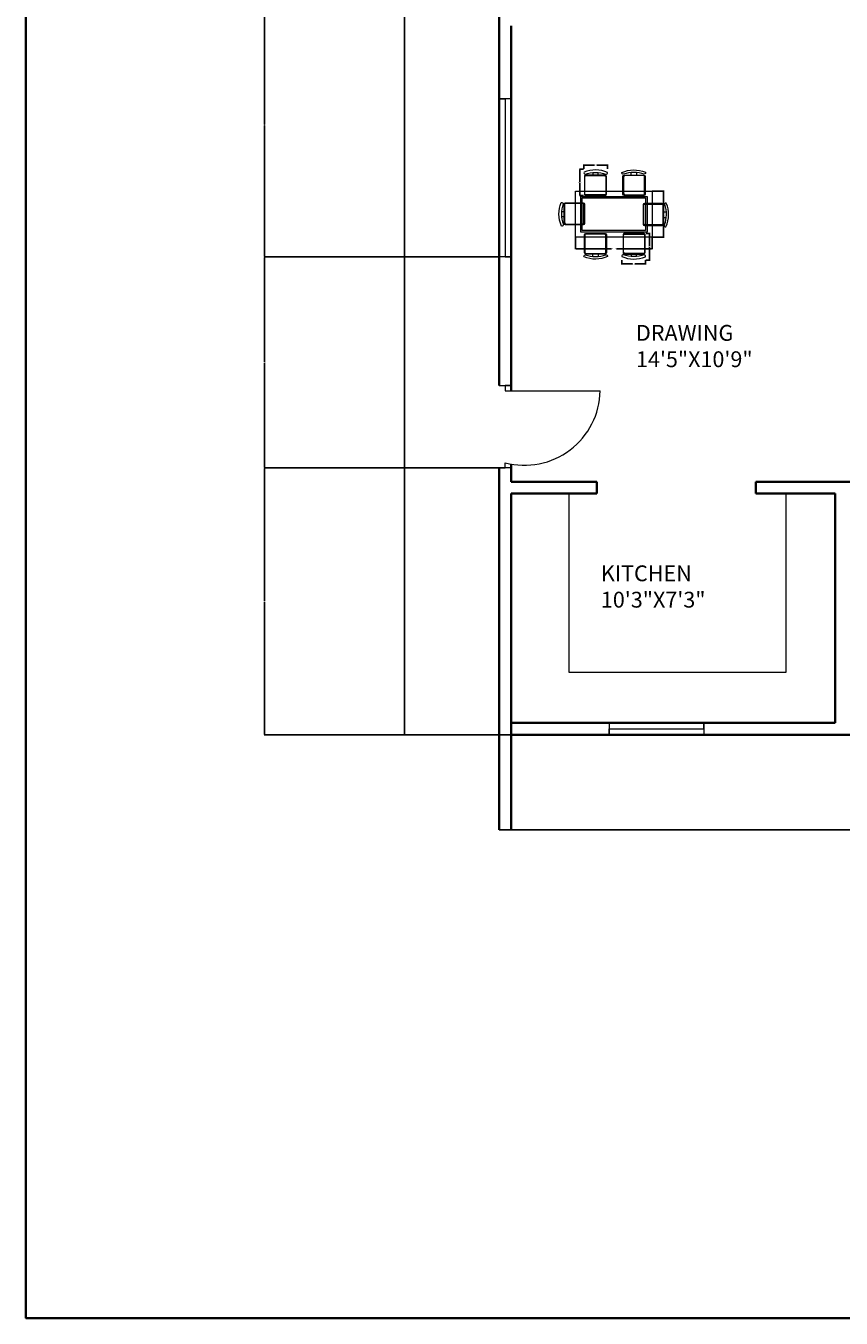
# Model space of a CAD drawing. Units: inches. Extents: x 1520 to 3401, y 1570 to 3432.
# Tile 1 of 15: x 1520 to 1829, y 1570 to 2061. Entities that reach past the tile are written whole.
import ezdxf

# ---------------------------------------------------------------- set-up
doc = ezdxf.new("R2010")
doc.units = ezdxf.units.IN
for name, color, linetype, lineweight in [('A-ANNO-DIMS', 2, 'Continuous', 18), ('A-ANNO-TTLB', 7, 'Continuous', 35), ('A-AREA-IDEN', 7, 'Continuous', 18), ('A-DOOR', 3, 'Continuous', 18), ('A-FLOR-CASE', 8, 'Continuous', 18), ('A-FLOR-EDGE', 7, 'Continuous', 25), ('A-FURN', 8, 'Continuous', 13), ('A-GLAZ', 4, 'Continuous', 18), ('A-WALL', 7, 'Continuous', 35)]:
    doc.layers.add(name, color=color, linetype=linetype, lineweight=lineweight)
doc.styles.get("Standard").update_dxf_attribs({"font": 'arial.ttf'})
doc.dimstyles.get("Standard").update_dxf_attribs({"dimtxt": 0.18, "dimasz": 0.18, "dimexe": 0.18, "dimexo": 0.0625, "dimgap": 0.09, "dimtad": 0, "dimtih": 1, "dimtoh": 1, "dimdec": 4, "dimzin": 0, "dimdsep": 46, "dimtxsty": 'Standard', "dimcen": 0.09, "dimadec": 0, "dimazin": 0, "dimtfac": 1, "dimtdec": 4, "dimtofl": 0, "dimtmove": 0, "dimatfit": 3, "dimfxl": 1, "dimtolj": 1, "dimtzin": 0, "dimarcsym": 0})

# ---------------------------------------------------------------- blocks, each defined once
blk = doc.blocks.new('DOOR-SWING-36-26')
for p, q in [((0, 31.26), (4.5, 31.26)), ((4.5, 31.26), (2.25, 31.26)), ((2.25, 31.26), (2.25, 29.26)), ((2.25, 29.26), (38.25, 29.26)), ((2.25, 0), (2.25, 2)), ((4.5, 0), (0, 0)), ((0, 0), (2.25, 0))]:
    blk.add_line(p, q)
blk.add_arc((9.61, 29.68), 28.64, 255.1135, 359.1603)
blk = doc.blocks.new('WIN-PLAN-60-02')
for p, q in [((4.5, 60), (0, 60)), ((0, 60), (2.25, 60)), ((2.25, 60), (2.25, 0)), ((4.5, 0), (0, 0)), ((2.25, 0), (4.5, 0))]:
    blk.add_line(p, q)
blk = doc.blocks.new('WIN-PLAN-36-04')
for p, q in [((0, 4.5), (0, 0)), ((0, 0), (0, 2.25)), ((0, 2.25), (36, 2.25)), ((36, 2.25), (36, 4.5)), ((36, 4.5), (36, 0))]:
    blk.add_line(p, q)
blk = doc.blocks.new('KITCHEN-COUNTER-01')
for p, q in [((0, 67.75), (0, 0)), ((82.51, 0), (82.51, 67.75)), ((0, 0), (82.51, 0))]:
    blk.add_line(p, q)
blk = doc.blocks.new('DINING-CHAIR-01')
for points in [[(0.47, 8.09, -0.175809), (8.38, 8.03, 0.578392), (8.97, 8.69, 0.214524), (0.06, 8.81, 0.552014), (0.47, 8.09, -0.065079)], [(8.04, 7.77), (0.7, 7.77, 0.414214), (0.19, 7.26), (0.19, 0.51, 0.414214), (0.7, 0), (8.04, 0, 0.414214), (8.55, 0.51), (8.55, 7.26, 0.414214), (8.04, 7.77)], [(5.46, 7.77), (5.46, 8.7, -0.064759)]]:
    blk.add_lwpolyline(points, format="xyb")
blk.add_lwpolyline([(0.71, 7.54), (7.81, 7.54, -0.414214), (8.32, 7.03), (8.32, 0.74, -0.414214), (7.81, 0.23), (0.71, 0.23, -0.512069), (0.42, 0.74), (0.42, 7.03, -0.512069)], format="xyb", close=True)
blk.add_lwpolyline([(3.41, 8.72), (3.41, 7.77)])
blk = doc.blocks.new('DINING-CHAIR-06')
for points in [[(8.29, 1.93, 0.414214), (8.81, 2.45), (8.81, 9.19, 0.414214), (8.29, 9.7), (0.96, 9.7, 0.414214), (0.45, 9.19), (0.45, 2.45, 0.414214), (0.96, 1.93), (8.29, 1.93)], [(8.52, 1.62, -0.175809), (0.62, 1.68, 0.578392), (0.02, 1.02, 0.214524), (8.94, 0.9, 0.552014), (8.52, 1.62, -0.065079)], [(3.53, 1.93), (3.53, 1, -0.064759)]]:
    blk.add_lwpolyline(points, format="xyb")
blk.add_lwpolyline([(8.29, 2.16), (1.19, 2.16, -0.414214), (0.68, 2.68), (0.68, 8.96, -0.414214), (1.19, 9.47), (8.29, 9.47, -0.512069), (8.58, 8.96), (8.58, 2.68, -0.512069)], format="xyb", close=True)
blk.add_lwpolyline([(5.59, 0.99), (5.59, 1.93)])
blk = doc.blocks.new('DINING-TABLE')
for points in [[(0, 17.41), (29.01, 17.41), (29.01, 0), (0, 0)], [(1.93, 15.47), (27.08, 15.47), (27.08, 1.93), (1.93, 1.93)], [(2.51, 14.89), (26.5, 14.89), (26.5, 2.51), (2.51, 2.51)]]:
    blk.add_lwpolyline(points, close=True)
blk = doc.blocks.new('*D175')
at = {"layer": 'A-ANNO-DIMS', "color": 0, "lineweight": -2, "transparency": 16777216}
for p, q in [((1731.63, 2006.36), (1730, 2006.36)), ((1730.18, 2006.18), (1730.18, 2001.52)), ((1730.18, 1996.49), (1730.18, 2001.15)), ((1731.63, 1996.31), (1730, 1996.31))]:
    blk.add_line(p, q, dxfattribs=at)
at = {"layer": 'A-ANNO-DIMS', "color": 0, "transparency": 16777216}
for points in [[(1730.15, 2006.18), (1730.21, 2006.18), (1730.18, 2006.36)], [(1730.15, 1996.49), (1730.21, 1996.49), (1730.18, 1996.31)]]:
    blk.add_solid(points, dxfattribs=at)
at = {"layer": 'Defpoints', "color": 0, "transparency": 16777216}
for p in [(1730.18, 2006.36), (1731.69, 2006.36), (1731.69, 1996.31)]:
    blk.add_point(p, dxfattribs=at)
at = {"layer": 'A-ANNO-DIMS', "color": 0, "transparency": 16777216, "insert": (1730.18, 2001.33), "char_height": 0.18, "attachment_point": 5}
blk.add_mtext('\\A1;CHAIR A 10 TYP.', dxfattribs=at)
blk = doc.blocks.new('*D176')
at = {"layer": 'A-ANNO-DIMS', "color": 0, "lineweight": -2, "transparency": 16777216}
for p, q in [((1731.69, 2006.42), (1731.69, 2008.04)), ((1731.87, 2007.86), (1735.76, 2007.86)), ((1740.56, 2007.86), (1736.67, 2007.86)), ((1740.74, 2006.42), (1740.74, 2008.04))]:
    blk.add_line(p, q, dxfattribs=at)
at = {"layer": 'A-ANNO-DIMS', "color": 0, "transparency": 16777216}
for points in [[(1731.87, 2007.89), (1731.87, 2007.83), (1731.69, 2007.86)], [(1740.56, 2007.89), (1740.56, 2007.83), (1740.74, 2007.86)]]:
    blk.add_solid(points, dxfattribs=at)
at = {"layer": 'Defpoints', "color": 0, "transparency": 16777216}
for p in [(1731.69, 2006.36), (1740.74, 2007.86), (1740.74, 2006.36)]:
    blk.add_point(p, dxfattribs=at)
at = {"layer": 'A-ANNO-DIMS', "color": 0, "transparency": 16777216, "insert": (1736.22, 2007.86), "char_height": 0.18, "attachment_point": 5}
blk.add_mtext('\\A1;9 TYP.', dxfattribs=at)
blk = doc.blocks.new('*D177')
at = {"layer": 'A-ANNO-DIMS', "color": 0, "lineweight": -2, "transparency": 16777216}
for p, q in [((1755.2, 1981.87), (1756.83, 1981.87)), ((1756.65, 1981.69), (1756.65, 1977.03)), ((1756.65, 1972.01), (1756.65, 1976.67)), ((1755.2, 1971.83), (1756.83, 1971.83))]:
    blk.add_line(p, q, dxfattribs=at)
at = {"layer": 'A-ANNO-DIMS', "color": 0, "transparency": 16777216}
for points in [[(1756.62, 1981.69), (1756.68, 1981.69), (1756.65, 1981.87)], [(1756.62, 1972.01), (1756.68, 1972.01), (1756.65, 1971.83)]]:
    blk.add_solid(points, dxfattribs=at)
at = {"layer": 'Defpoints', "color": 0, "transparency": 16777216}
for p in [(1755.14, 1981.87), (1756.65, 1981.87), (1755.14, 1971.83)]:
    blk.add_point(p, dxfattribs=at)
at = {"layer": 'A-ANNO-DIMS', "color": 0, "transparency": 16777216, "insert": (1756.65, 1976.85), "char_height": 0.18, "attachment_point": 5}
blk.add_mtext('\\A1;CHAIR B 10 TYP.', dxfattribs=at)
blk = doc.blocks.new('*D178')
at = {"layer": 'A-ANNO-DIMS', "color": 0, "lineweight": -2, "transparency": 16777216}
for p, q in [((1746.09, 1971.77), (1746.09, 1970.14)), ((1755.14, 1971.77), (1755.14, 1970.14)), ((1746.27, 1970.32), (1750.15, 1970.32)), ((1754.96, 1970.32), (1751.07, 1970.32))]:
    blk.add_line(p, q, dxfattribs=at)
at = {"layer": 'A-ANNO-DIMS', "color": 0, "transparency": 16777216}
for points in [[(1746.27, 1970.35), (1746.27, 1970.29), (1746.09, 1970.32)], [(1754.96, 1970.35), (1754.96, 1970.29), (1755.14, 1970.32)]]:
    blk.add_solid(points, dxfattribs=at)
at = {"layer": 'Defpoints', "color": 0, "transparency": 16777216}
for p in [(1746.09, 1971.83), (1755.14, 1971.83), (1755.14, 1970.32)]:
    blk.add_point(p, dxfattribs=at)
at = {"layer": 'A-ANNO-DIMS', "color": 0, "transparency": 16777216, "insert": (1750.61, 1970.32), "char_height": 0.18, "attachment_point": 5}
blk.add_mtext('\\A1;9 TYP.', dxfattribs=at)
blk = doc.blocks.new('*D179')
at = {"layer": 'A-ANNO-DIMS', "color": 0, "lineweight": -2, "transparency": 16777216}
for p, q in [((1728.6, 1980.42), (1728.6, 1975.95)), ((1728.78, 1976.13), (1742.14, 1976.13)), ((1757.43, 1976.13), (1744.07, 1976.13)), ((1757.61, 1980.42), (1757.61, 1975.95))]:
    blk.add_line(p, q, dxfattribs=at)
at = {"layer": 'A-ANNO-DIMS', "color": 0, "transparency": 16777216}
for points in [[(1728.78, 1976.16), (1728.78, 1976.1), (1728.6, 1976.13)], [(1757.43, 1976.16), (1757.43, 1976.1), (1757.61, 1976.13)]]:
    blk.add_solid(points, dxfattribs=at)
at = {"layer": 'Defpoints', "color": 0, "transparency": 16777216}
for p in [(1728.6, 1980.48), (1757.61, 1980.48), (1757.61, 1976.13)]:
    blk.add_point(p, dxfattribs=at)
at = {"layer": 'A-ANNO-DIMS', "color": 0, "transparency": 16777216, "insert": (1743.1, 1976.13), "char_height": 0.18, "attachment_point": 5}
blk.add_mtext('\\A1;TABLE 29 TYP.', dxfattribs=at)
blk = doc.blocks.new('*D180')
at = {"layer": 'A-ANNO-DIMS', "color": 0, "lineweight": -2, "transparency": 16777216}
for p, q in [((1757.67, 1997.89), (1762.14, 1997.89)), ((1761.96, 1997.71), (1761.96, 1989.37)), ((1761.96, 1980.66), (1761.96, 1989)), ((1757.67, 1980.48), (1762.14, 1980.48))]:
    blk.add_line(p, q, dxfattribs=at)
at = {"layer": 'A-ANNO-DIMS', "color": 0, "transparency": 16777216}
for points in [[(1761.93, 1997.71), (1761.99, 1997.71), (1761.96, 1997.89)], [(1761.93, 1980.66), (1761.99, 1980.66), (1761.96, 1980.48)]]:
    blk.add_solid(points, dxfattribs=at)
at = {"layer": 'Defpoints', "color": 0, "transparency": 16777216}
for p in [(1757.61, 1997.89), (1761.96, 1997.89), (1757.61, 1980.48)]:
    blk.add_point(p, dxfattribs=at)
at = {"layer": 'A-ANNO-DIMS', "color": 0, "transparency": 16777216, "insert": (1761.96, 1989.19), "char_height": 0.18, "attachment_point": 5}
blk.add_mtext('\\A1;17 TYP.', dxfattribs=at)
blk = doc.blocks.new('*D185')
at = {"layer": 'A-ANNO-DIMS', "color": 0, "lineweight": -2, "transparency": 16777216}
for p, q in [((1699.55, 1892.93), (1610.33, 1892.93)), ((1610.51, 1892.75), (1610.51, 1842.49)), ((1610.51, 1791.86), (1610.51, 1842.12)), ((1704.05, 1791.68), (1610.33, 1791.68))]:
    blk.add_line(p, q, dxfattribs=at)
at = {"layer": 'A-ANNO-DIMS', "color": 0, "transparency": 16777216}
for points in [[(1610.48, 1892.75), (1610.54, 1892.75), (1610.51, 1892.93)], [(1610.48, 1791.86), (1610.54, 1791.86), (1610.51, 1791.68)]]:
    blk.add_solid(points, dxfattribs=at)
at = {"layer": 'Defpoints', "color": 0, "transparency": 16777216}
for p in [(1610.51, 1892.93), (1699.61, 1892.93), (1704.11, 1791.68)]:
    blk.add_point(p, dxfattribs=at)
at = {"layer": 'A-ANNO-DIMS', "color": 0, "transparency": 16777216, "insert": (1610.51, 1842.31), "char_height": 0.18, "attachment_point": 5}
blk.add_mtext('\\A1;101.26', dxfattribs=at)
blk = doc.blocks.new('*D186')
at = {"layer": 'A-ANNO-DIMS', "color": 0, "lineweight": -2, "transparency": 16777216}
for p, q in [((1699.55, 1973), (1610.33, 1973)), ((1610.51, 1972.82), (1610.51, 1933.15)), ((1610.51, 1893.11), (1610.51, 1932.79)), ((1699.55, 1892.93), (1610.33, 1892.93))]:
    blk.add_line(p, q, dxfattribs=at)
at = {"layer": 'A-ANNO-DIMS', "color": 0, "transparency": 16777216}
for points in [[(1610.48, 1972.82), (1610.54, 1972.82), (1610.51, 1973)], [(1610.48, 1893.11), (1610.54, 1893.11), (1610.51, 1892.93)]]:
    blk.add_solid(points, dxfattribs=at)
at = {"layer": 'Defpoints', "color": 0, "transparency": 16777216}
for p in [(1610.51, 1973), (1699.61, 1973), (1699.61, 1892.93)]:
    blk.add_point(p, dxfattribs=at)
at = {"layer": 'A-ANNO-DIMS', "color": 0, "transparency": 16777216, "insert": (1610.51, 1932.97), "char_height": 0.18, "attachment_point": 5}
blk.add_mtext('\\A1;80.07', dxfattribs=at)
blk = doc.blocks.new('*D187')
at = {"layer": 'A-ANNO-DIMS', "color": 0, "lineweight": -2, "transparency": 16777216}
for p, q in [((1699.55, 2073.12), (1610.33, 2073.12)), ((1610.51, 2072.94), (1610.51, 2023.24)), ((1610.51, 1973.18), (1610.51, 2022.88)), ((1699.55, 1973), (1610.33, 1973))]:
    blk.add_line(p, q, dxfattribs=at)
at = {"layer": 'A-ANNO-DIMS', "color": 0, "transparency": 16777216}
for points in [[(1610.48, 2072.94), (1610.54, 2072.94), (1610.51, 2073.12)], [(1610.48, 1973.18), (1610.54, 1973.18), (1610.51, 1973)]]:
    blk.add_solid(points, dxfattribs=at)
at = {"layer": 'Defpoints', "color": 0, "transparency": 16777216}
for p in [(1610.51, 2073.12), (1699.61, 2073.12), (1699.61, 1973)]:
    blk.add_point(p, dxfattribs=at)
at = {"layer": 'A-ANNO-DIMS', "color": 0, "transparency": 16777216, "insert": (1610.51, 2023.06), "char_height": 0.18, "attachment_point": 5}
blk.add_mtext('\\A1;100.12', dxfattribs=at)

msp = doc.modelspace()

# ---------------------------------------------------------------- linework, layer by layer
at = {"layer": 'A-ANNO-TTLB'}
msp.add_lwpolyline([(1519.9253, 3431.7421), (3400.8761, 3431.7421), (3400.8761, 1570.3458), (1519.9253, 1570.3458)], close=True, dxfattribs=at)
at = {"layer": 'A-FLOR-EDGE'}
for p, q in [((1663.6128, 2733.1786), (1663.6128, 1791.6786)), ((1704.1128, 1791.6786), (1663.6128, 1791.6786)), ((1704.1128, 1791.6786), (1704.1128, 1755.6786)), ((1699.6128, 1755.6786), (2339.6128, 1755.6786))]:
    msp.add_line(p, q, dxfattribs=at)
at = {"layer": 'A-FURN'}
for points in [[(1746.741, 2004.3409, -0.57839206), (1746.1424, 2004.9991, -0.21452438), (1755.0618, 2005.1188, -0.55201397), (1754.6427, 2004.4007, 0.1758092), (1746.741, 2004.3409)], [(1754.4119, 2004.0836, -0.41421356), (1754.9252, 2003.5704), (1754.9252, 1996.8254, -0.41421356), (1754.4119, 1996.3122), (1747.0763, 1996.3122, -0.41421356), (1746.5631, 1996.8254), (1746.5631, 2003.5704, -0.41421356), (1747.0763, 2004.0836), (1754.4119, 2004.0836)], [(1749.6529, 2004.0836), (1749.6529, 2005.0113, 0.06475861)], [(1723.9204, 1985.3193, -0.57839206), (1723.2622, 1984.7207, -0.21452438), (1723.1425, 1993.6401, -0.55201397), (1723.8606, 1993.221, 0.17580937), (1723.9204, 1985.3193)], [(1724.1777, 1992.9902, -0.41421356), (1724.6909, 1993.5034), (1731.436, 1993.5034, -0.41421356), (1731.9492, 1992.9902), (1731.9492, 1985.6546, -0.41421356), (1731.436, 1985.1413), (1724.6909, 1985.1413, -0.41421356), (1724.1777, 1985.6546), (1724.1777, 1992.9902)], [(1761.953, 1992.739, 0.41421356), (1761.4398, 1993.2522), (1754.6948, 1993.2522, 0.41421356), (1754.1816, 1992.739), (1754.1816, 1985.4033, 0.41421356), (1754.6948, 1984.8901), (1761.4398, 1984.8901, 0.41421356), (1761.953, 1985.4033), (1761.953, 1992.739)], [(1762.2702, 1992.9698, -0.17580919), (1762.2103, 1985.0681, 0.57839206), (1762.8685, 1984.4695, 0.21452438), (1762.9882, 1993.3888, 0.55201397), (1762.2701, 1992.9698, -0.06507904)], [(1724.1777, 1988.2312), (1723.25, 1988.2312, 0.06475861)], [(1761.953, 1987.98), (1762.8807, 1987.98, -0.06475861)], [(1739.7536, 1974.1004), (1732.4179, 1974.1004, -0.41421356), (1731.9047, 1974.6136), (1731.9047, 1981.3586, -0.41421356), (1732.4179, 1981.8718), (1739.7536, 1981.8718, -0.41421356), (1740.2668, 1981.3586), (1740.2668, 1974.6136, -0.41421356), (1739.7536, 1974.1004)], [(1740.0888, 1973.8431, -0.57839206), (1740.6874, 1973.1848, -0.21452438), (1731.7681, 1973.0652, -0.55201397), (1732.1871, 1973.7832, 0.17580929), (1740.0888, 1973.8431)], [(1737.1769, 1974.1004), (1737.1769, 1973.1726, 0.06475861)]]:
    msp.add_lwpolyline(points, format="xyb", dxfattribs=at)
for points in [[(1754.4088, 2003.8524), (1747.3075, 2003.8524, 0.41421356), (1746.7943, 2003.3392), (1746.7943, 1997.0566, 0.41421356), (1747.3075, 1996.5434), (1754.4088, 1996.5434, 0.51206948), (1754.694, 1997.0566), (1754.694, 2003.3392, 0.51206948)], [(1724.4089, 1992.9871), (1724.4089, 1985.8858, 0.41421356), (1724.9221, 1985.3725), (1731.2047, 1985.3725, 0.41421356), (1731.718, 1985.8858), (1731.718, 1992.9871, 0.51206948), (1731.2047, 1993.2722), (1724.9221, 1993.2722, 0.51206948)], [(1761.7218, 1992.7359), (1761.7218, 1985.6345, -0.41421356), (1761.2086, 1985.1213), (1754.926, 1985.1213, -0.41421356), (1754.4128, 1985.6345), (1754.4128, 1992.7359, -0.51206948), (1754.926, 1993.021), (1761.2086, 1993.021, -0.51206948)], [(1732.421, 1974.3316), (1739.5224, 1974.3316, 0.41421356), (1740.0356, 1974.8448), (1740.0356, 1981.1274, 0.41421356), (1739.5224, 1981.6406), (1732.421, 1981.6406, 0.51206948), (1732.1359, 1981.1274), (1732.1359, 1974.8448, 0.51206948)]]:
    msp.add_lwpolyline(points, format="xyb", close=True, dxfattribs=at)
for points in [[(1751.7063, 2005.0282), (1751.7063, 2004.0836)], [(1723.2331, 1990.2846), (1724.1777, 1990.2846)], [(1762.8976, 1990.0333), (1761.953, 1990.0333)], [(1735.1236, 1973.1558), (1735.1236, 1974.1004)]]:
    msp.add_lwpolyline(points, dxfattribs=at)
at = {"layer": 'A-WALL'}
for p, q in [((1699.6128, 2075.1195), (1699.6128, 1924.1968)), ((1699.6128, 2075.1195), (1699.6128, 1924.1968)), ((1704.1128, 2060.6786), (1704.1128, 1922.1968)), ((1699.6128, 1892.9337), (1699.6128, 1755.6786)), ((1699.6128, 1892.9337), (1699.6128, 1755.6786)), ((1704.1128, 1894.4316), (1704.1128, 1887.6786)), ((1736.6742, 1887.6786), (1704.1128, 1887.6786)), ((1704.1128, 1883.1786), (1704.1128, 1755.6786)), ((1736.6742, 1883.1786), (1704.1128, 1883.1786)), ((1736.6742, 1883.1786), (1736.6742, 1887.6786)), ((1796.9488, 1883.1786), (1796.9488, 1887.6786)), ((1857.4148, 1887.6786), (1796.9488, 1887.6786)), ((1827.1128, 1883.1786), (1796.9488, 1883.1786)), ((1827.1128, 1883.1786), (1827.1128, 1796.1786)), ((1827.1128, 1796.1786), (1704.1128, 1796.1786)), ((1896.7277, 1791.6786), (1704.1128, 1791.6786))]:
    msp.add_line(p, q, dxfattribs=at)

# ---------------------------------------------------------------- block references
at = {"layer": 'A-DOOR'}
msp.add_blockref('DOOR-SWING-36-26', (1699.613, 1892.934), dxfattribs=at)
at = {"layer": 'A-FLOR-CASE'}
msp.add_blockref('KITCHEN-COUNTER-01', (1726.006, 1815.432), dxfattribs=at)
at = {"layer": 'A-FURN'}
for name, p in [('DINING-CHAIR-01', (1731.713, 1996.312)), ('DINING-TABLE', (1728.599, 1980.482)), ('DINING-CHAIR-06', (1746.118, 1972.168))]:
    msp.add_blockref(name, p, dxfattribs=at)
at = {"layer": 'A-GLAZ'}
for name, p in [('WIN-PLAN-60-02', (1699.613, 1973.002)), ('WIN-PLAN-36-04', (1741.2965, 1791.679))]:
    msp.add_blockref(name, p, dxfattribs=at)

# ---------------------------------------------------------------- texts
at = {"layer": 'A-AREA-IDEN', "char_height": 6, "attachment_point": 1}
for s, width, insert in [('DRAWING\\P14\'5"X10\'9"', 109.875241, (1751.4939, 1947.185)), ('KITCHEN\\P10\'3"X7\'3"', 147.450562, (1738.1623, 1855.9523))]:
    msp.add_mtext_dynamic_manual_height_columns(s, width=width, gutter_width=12.5, heights=[0], dxfattribs=dict(at, insert=insert))

# ---------------------------------------------------------------- dimensions: what is measured, and where the dimension line sits
at = {"layer": 'A-ANNO-DIMS'}
for base, p1, p2, picture, middle in [((1610.5128, 2073.1195), (1699.6128, 1973.0015), (1699.6128, 2073.1195), '*D187', (1610.5128, 2023.0605)), ((1610.5128, 1973.0015), (1699.6128, 1892.9337), (1699.6128, 1973.0015), '*D186', (1610.5128, 1932.9676)), ((1610.5128, 1892.9337), (1704.1128, 1791.6786), (1699.6128, 1892.9337), '*D185', (1610.5128, 1842.3062))]:
    dim = msp.add_linear_dim(base=base, p1=p1, p2=p2, angle=90, dimstyle='Standard', override={"dimdec": 2, "dimlfac": 1, "dimrnd": 0, "dimzin": 0, "dimdsep": 46, "dimlunit": 2}, dxfattribs=at)
    dim.commit()
    dim.dimension.update_dxf_attribs({"geometry": picture, "text_midpoint": middle})
for base, p1, p2, text, picture, middle in [((1730.1834, 2006.3563), (1731.6901, 1996.3122), (1731.6901, 2006.3563), 'CHAIR A <> TYP.', '*D175', (1730.1834, 2001.3343)), ((1761.9611, 1997.8884), (1757.6095, 1980.482), (1757.6095, 1997.8884), '<> TYP.', '*D180', (1761.9611, 1989.1852)), ((1756.6464, 1981.8718), (1755.1398, 1971.8276), (1755.1398, 1981.8718), 'CHAIR B <> TYP.', '*D177', (1756.6464, 1976.8497))]:
    dim = msp.add_linear_dim(base=base, p1=p1, p2=p2, angle=90, text=text, dimstyle='Standard', override={"dimdec": 0, "dimlfac": 1, "dimrnd": 0, "dimzin": 0, "dimdsep": 46, "dimlunit": 2}, dxfattribs=at)
    dim.commit()
    dim.dimension.update_dxf_attribs({"geometry": picture, "text_midpoint": middle})
for base, p1, p2, text, picture, middle in [((1740.7436, 2007.863), (1731.6901, 2006.3563), (1740.7436, 2006.3563), '<> TYP.', '*D176', (1736.2168, 2007.863)), ((1757.6095, 1976.1304), (1728.5988, 1980.482), (1757.6095, 1980.482), 'TABLE <> TYP.', '*D179', (1743.1042, 1976.1304)), ((1755.1398, 1970.321), (1746.0863, 1971.8276), (1755.1398, 1971.8276), '<> TYP.', '*D178', (1750.613, 1970.321))]:
    dim = msp.add_linear_dim(base=base, p1=p1, p2=p2, text=text, dimstyle='Standard', override={"dimdec": 0, "dimlfac": 1, "dimrnd": 0, "dimzin": 0, "dimdsep": 46, "dimlunit": 2}, dxfattribs=at)
    dim.commit()
    dim.dimension.update_dxf_attribs({"geometry": picture, "text_midpoint": middle})

doc.saveas('drawing.dxf')
